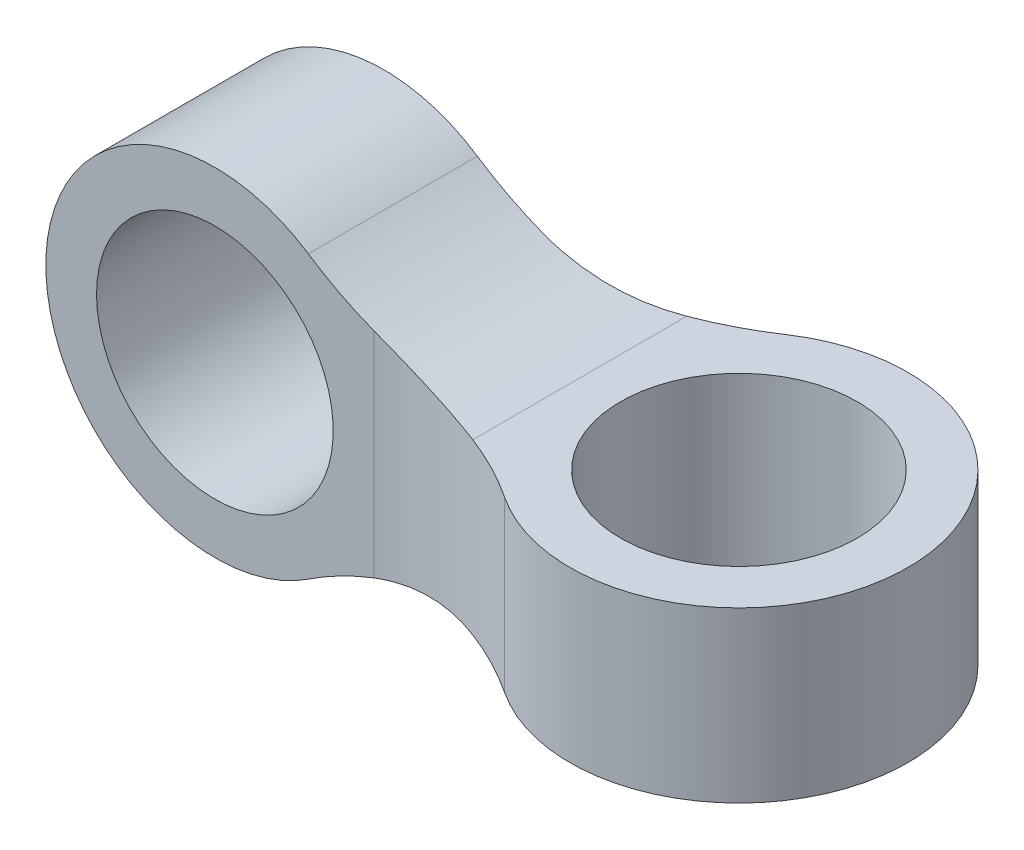
ISO-10303-21;
HEADER;
FILE_DESCRIPTION(('STEP AP214'),'2;1');
FILE_NAME('part.step','',(''),(''),'','','');
FILE_SCHEMA(('AUTOMOTIVE_DESIGN { 1 0 10303 214 1 1 1 1 }'));
ENDSEC;
DATA;
#1=APPLICATION_CONTEXT('core data for automotive mechanical design processes');
#2=APPLICATION_PROTOCOL_DEFINITION('international standard','automotive_design',2000,#1);
#3=PRODUCT_CONTEXT('',#1,'mechanical');
#4=PRODUCT('Part','Part','',(#3));
#5=PRODUCT_RELATED_PRODUCT_CATEGORY('part','',(#4));
#6=PRODUCT_DEFINITION_FORMATION('','',#4);
#7=PRODUCT_DEFINITION_CONTEXT('part definition',#1,'design');
#8=PRODUCT_DEFINITION('design','',#6,#7);
#9=PRODUCT_DEFINITION_SHAPE('','',#8);
#10=(LENGTH_UNIT() NAMED_UNIT(*) SI_UNIT(.MILLI.,.METRE.));
#11=(NAMED_UNIT(*) PLANE_ANGLE_UNIT() SI_UNIT($,.RADIAN.));
#12=(NAMED_UNIT(*) SI_UNIT($,.STERADIAN.) SOLID_ANGLE_UNIT());
#13=UNCERTAINTY_MEASURE_WITH_UNIT(LENGTH_MEASURE(1.E-05),#10,'distance_accuracy_value','');
#14=(GEOMETRIC_REPRESENTATION_CONTEXT(3) GLOBAL_UNCERTAINTY_ASSIGNED_CONTEXT((#13)) GLOBAL_UNIT_ASSIGNED_CONTEXT((#10,
#11,#12)) REPRESENTATION_CONTEXT('',''));
#15=CARTESIAN_POINT('',(0.,0.,0.));
#16=DIRECTION('',(0.,0.,1.));
#17=DIRECTION('',(1.,0.,0.));
#18=AXIS2_PLACEMENT_3D('',#15,#16,#17);
#19=CARTESIAN_POINT('',(-13.,0.,-25.));
#20=DIRECTION('',(0.,0.,1.));
#21=DIRECTION('',(1.,0.,0.));
#22=AXIS2_PLACEMENT_3D('',#19,#20,#21);
#23=CYLINDRICAL_SURFACE('',#22,10.);
#24=CARTESIAN_POINT('',(-13.,0.,5.));
#25=DIRECTION('',(0.,0.,-1.));
#26=DIRECTION('',(-1.,0.,0.));
#27=AXIS2_PLACEMENT_3D('',#24,#25,#26);
#28=CIRCLE('',#27,10.);
#29=CARTESIAN_POINT('',(-7.47229201607434,8.33333333333333,5.));
#30=VERTEX_POINT('',#29);
#31=CARTESIAN_POINT('',(-7.47229201607434,-8.33333333333333,5.));
#32=VERTEX_POINT('',#31);
#33=EDGE_CURVE('E345',#30,#32,#28,.F.);
#34=ORIENTED_EDGE('',*,*,#33,.F.);
#35=DIRECTION('',(0.,0.,1.));
#36=VECTOR('',#35,1.);
#37=CARTESIAN_POINT('',(-7.47229201607434,8.33333333333333,-25.));
#38=LINE('',#37,#36);
#39=CARTESIAN_POINT('',(-7.47229201607434,8.33333333333333,-5.));
#40=VERTEX_POINT('',#39);
#41=EDGE_CURVE('E310',#40,#30,#38,.T.);
#42=ORIENTED_EDGE('',*,*,#41,.F.);
#43=CARTESIAN_POINT('',(-13.,0.,-5.));
#44=DIRECTION('',(0.,0.,-1.));
#45=DIRECTION('',(-1.,0.,0.));
#46=AXIS2_PLACEMENT_3D('',#43,#44,#45);
#47=CIRCLE('',#46,10.);
#48=CARTESIAN_POINT('',(-7.47229201607434,-8.33333333333333,-5.));
#49=VERTEX_POINT('',#48);
#50=EDGE_CURVE('E233',#40,#49,#47,.F.);
#51=ORIENTED_EDGE('',*,*,#50,.T.);
#52=DIRECTION('',(0.,0.,1.));
#53=VECTOR('',#52,1.);
#54=CARTESIAN_POINT('',(-7.47229201607434,-8.33333333333333,-25.));
#55=LINE('',#54,#53);
#56=EDGE_CURVE('E301',#49,#32,#55,.T.);
#57=ORIENTED_EDGE('',*,*,#56,.T.);
#58=EDGE_LOOP('',(#34,#42,#51,#57));
#59=FACE_BOUND('',#58,.T.);
#60=ADVANCED_FACE('F165',(#59),#23,.T.);
#61=CARTESIAN_POINT('',(0.,5.,-25.));
#62=DIRECTION('',(0.,-1.,0.));
#63=DIRECTION('',(1.,0.,0.));
#64=AXIS2_PLACEMENT_3D('',#61,#62,#63);
#65=PLANE('',#64);
#66=CARTESIAN_POINT('',(13.,5.,0.));
#67=DIRECTION('',(0.,-1.,0.));
#68=DIRECTION('',(1.,0.,0.));
#69=AXIS2_PLACEMENT_3D('',#66,#67,#68);
#70=CIRCLE('',#69,7.);
#71=CARTESIAN_POINT('',(20.,5.,0.));
#72=VERTEX_POINT('',#71);
#73=EDGE_CURVE('E324',#72,#72,#70,.T.);
#74=ORIENTED_EDGE('',*,*,#73,.T.);
#75=EDGE_LOOP('',(#74));
#76=FACE_BOUND('',#75,.T.);
#77=CARTESIAN_POINT('',(-3.583123951777,5.,25.));
#78=DIRECTION('',(0.,-1.,0.));
#79=DIRECTION('',(1.,0.,0.));
#80=AXIS2_PLACEMENT_3D('',#77,#78,#79);
#81=CIRCLE('',#80,20.);
#82=CARTESIAN_POINT('',(7.47229201607434,5.,8.33333333333334));
#83=VERTEX_POINT('',#82);
#84=CARTESIAN_POINT('',(3.58312395177704,4.99999999999995,6.32796500151069));
#85=VERTEX_POINT('',#84);
#86=EDGE_CURVE('E177',#83,#85,#81,.F.);
#87=ORIENTED_EDGE('',*,*,#86,.F.);
#88=CARTESIAN_POINT('',(13.,5.,0.));
#89=DIRECTION('',(0.,-1.,0.));
#90=DIRECTION('',(1.,0.,0.));
#91=AXIS2_PLACEMENT_3D('',#88,#89,#90);
#92=CIRCLE('',#91,10.);
#93=CARTESIAN_POINT('',(7.47229201607433,5.,-8.33333333333333));
#94=VERTEX_POINT('',#93);
#95=EDGE_CURVE('E256',#94,#83,#92,.T.);
#96=ORIENTED_EDGE('',*,*,#95,.F.);
#97=CARTESIAN_POINT('',(-3.583123951777,5.,-25.));
#98=DIRECTION('',(0.,-1.,0.));
#99=DIRECTION('',(1.,0.,0.));
#100=AXIS2_PLACEMENT_3D('',#97,#98,#99);
#101=CIRCLE('',#100,20.);
#102=CARTESIAN_POINT('',(3.58312395177704,4.99999999999995,-6.32796500151069));
#103=VERTEX_POINT('',#102);
#104=EDGE_CURVE('E254',#94,#103,#101,.T.);
#105=ORIENTED_EDGE('',*,*,#104,.T.);
#106=DIRECTION('',(0.,0.,1.));
#107=VECTOR('',#106,1.);
#108=CARTESIAN_POINT('',(3.58312395177699,5.,-25.));
#109=LINE('',#108,#107);
#110=EDGE_CURVE('E255',#103,#85,#109,.T.);
#111=ORIENTED_EDGE('',*,*,#110,.T.);
#112=EDGE_LOOP('',(#87,#96,#105,#111));
#113=FACE_BOUND('',#112,.T.);
#114=ADVANCED_FACE('F349',(#76,#113),#65,.F.);
#115=CARTESIAN_POINT('',(3.58312395177699,25.,-25.));
#116=DIRECTION('',(0.,0.,1.));
#117=DIRECTION('',(1.,0.,0.));
#118=AXIS2_PLACEMENT_3D('',#115,#116,#117);
#119=CYLINDRICAL_SURFACE('',#118,20.);
#120=CARTESIAN_POINT('',(7.47229201607434,5.38178469463521,8.33333333333333));
#121=CARTESIAN_POINT('',(7.29699032317259,5.34703236946405,8.21705135141738));
#122=CARTESIAN_POINT('',(7.11958800828395,5.31430622195632,8.10335941718668));
#123=CARTESIAN_POINT('',(6.76071891900881,5.2532019543182,7.88131271793948));
#124=CARTESIAN_POINT('',(6.57925177284516,5.22482423377966,7.7729584440389));
#125=CARTESIAN_POINT('',(6.02882561809351,5.14664056772693,7.45606457285716));
#126=CARTESIAN_POINT('',(5.6540157645712,5.1038191206325,7.25580939391501));
#127=CARTESIAN_POINT('',(4.88995933117876,5.03904902020734,6.8784966546735));
#128=CARTESIAN_POINT('',(4.50067842728979,5.01715378266823,6.70149944909328));
#129=CARTESIAN_POINT('',(3.71110175343317,4.99651277313733,6.37267960841244));
#130=CARTESIAN_POINT('',(3.31080898852315,4.99776074689242,6.22085018312637));
#131=CARTESIAN_POINT('',(2.50015157937633,5.02520585072317,5.94276436337308));
#132=CARTESIAN_POINT('',(2.08974859443147,5.05151960391396,5.81663085531488));
#133=CARTESIAN_POINT('',(1.26396259082839,5.13058788823112,5.59152465950283));
#134=CARTESIAN_POINT('',(0.848578641653094,5.18334743736802,5.49255713193));
#135=CARTESIAN_POINT('',(0.0177355960030123,5.31588247949777,5.3222677787619));
#136=CARTESIAN_POINT('',(-0.397719870811708,5.39558008538139,5.25086750767909));
#137=CARTESIAN_POINT('',(-1.22607394668929,5.58218052923217,5.13497842084868));
#138=CARTESIAN_POINT('',(-1.63897376743929,5.68906927003721,5.09047570038574));
#139=CARTESIAN_POINT('',(-2.30757201952622,5.88528115160457,5.03902874204332));
#140=CARTESIAN_POINT('',(-2.56509330773308,5.96654705369896,5.02428612595834));
#141=CARTESIAN_POINT('',(-3.07676594844552,6.13949048658364,5.00477143854931));
#142=CARTESIAN_POINT('',(-3.33091988173299,6.23115945884189,4.99999123302929));
#143=CARTESIAN_POINT('',(-3.583123951777,6.32796500151074,5.));
#144=B_SPLINE_CURVE_WITH_KNOTS('',3,(#120,#121,#122,#123,#124,#125,#126,#127,#128,#129,#130,
#131,#132,#133,#134,#135,#136,#137,#138,#139,#140,#141,#142,#143),.UNSPECIFIED.,.F.,.F.,(4,2,2,
2,2,2,2,2,2,2,2,4),(0.,0.639568646578073,1.27919603010921,2.55908404816412,3.84223042353997,
5.12503004473554,6.41382742723958,7.70286944781018,8.98821584478183,10.2728972110752,
11.083848336485,11.8941370696184),.UNSPECIFIED.);
#145=CARTESIAN_POINT('',(-3.583123951777,6.32796500151074,5.));
#146=VERTEX_POINT('',#145);
#147=EDGE_CURVE('E296',#85,#146,#144,.T.);
#148=ORIENTED_EDGE('',*,*,#147,.F.);
#149=ORIENTED_EDGE('',*,*,#110,.F.);
#150=CARTESIAN_POINT('',(7.47229201607433,5.3817846946352,-8.33333333333334));
#151=CARTESIAN_POINT('',(7.29699032317258,5.34703236946404,-8.21705135141739));
#152=CARTESIAN_POINT('',(7.11958800828394,5.31430622195631,-8.10335941718669));
#153=CARTESIAN_POINT('',(6.7607189190088,5.2532019543182,-7.88131271793948));
#154=CARTESIAN_POINT('',(6.57925177284515,5.22482423377965,-7.7729584440389));
#155=CARTESIAN_POINT('',(6.0288256180935,5.14664056772693,-7.45606457285716));
#156=CARTESIAN_POINT('',(5.6540157645712,5.1038191206325,-7.25580939391501));
#157=CARTESIAN_POINT('',(4.88995933117876,5.03904902020734,-6.8784966546735));
#158=CARTESIAN_POINT('',(4.50067842728979,5.01715378266822,-6.70149944909328));
#159=CARTESIAN_POINT('',(3.71110175343317,4.99651277313733,-6.37267960841245));
#160=CARTESIAN_POINT('',(3.31080898852315,4.99776074689242,-6.22085018312637));
#161=CARTESIAN_POINT('',(2.50015157937632,5.02520585072317,-5.94276436337308));
#162=CARTESIAN_POINT('',(2.08974859443147,5.05151960391397,-5.81663085531489));
#163=CARTESIAN_POINT('',(1.26396259082839,5.13058788823112,-5.59152465950283));
#164=CARTESIAN_POINT('',(0.848578641653089,5.18334743736802,-5.49255713193001));
#165=CARTESIAN_POINT('',(0.0177355960030073,5.31588247949777,-5.3222677787619));
#166=CARTESIAN_POINT('',(-0.397719870811712,5.39558008538139,-5.25086750767909));
#167=CARTESIAN_POINT('',(-1.22607394668929,5.58218052923217,-5.13497842084869));
#168=CARTESIAN_POINT('',(-1.63897376743929,5.68906927003722,-5.09047570038574));
#169=CARTESIAN_POINT('',(-2.30757201952623,5.88528115160457,-5.03902874204333));
#170=CARTESIAN_POINT('',(-2.56509330773309,5.96654705369896,-5.02428612595834));
#171=CARTESIAN_POINT('',(-3.07676594844552,6.13949048658364,-5.00477143854931));
#172=CARTESIAN_POINT('',(-3.330919881733,6.23115945884189,-4.9999912330293));
#173=CARTESIAN_POINT('',(-3.583123951777,6.32796500151074,-5.));
#174=B_SPLINE_CURVE_WITH_KNOTS('',3,(#150,#151,#152,#153,#154,#155,#156,#157,#158,#159,#160,
#161,#162,#163,#164,#165,#166,#167,#168,#169,#170,#171,#172,#173),.UNSPECIFIED.,.F.,.F.,(4,2,2,
2,2,2,2,2,2,2,2,4),(0.,0.639568646578075,1.27919603010921,2.55908404816412,3.84223042353997,
5.12503004473554,6.41382742723958,7.70286944781018,8.98821584478183,10.2728972110752,
11.083848336485,11.8941370696184),.UNSPECIFIED.);
#175=CARTESIAN_POINT('',(-3.583123951777,6.32796500151074,-5.));
#176=VERTEX_POINT('',#175);
#177=EDGE_CURVE('E244',#103,#176,#174,.T.);
#178=ORIENTED_EDGE('',*,*,#177,.T.);
#179=CARTESIAN_POINT('',(3.58312395177699,25.,-5.));
#180=DIRECTION('',(0.,0.,-1.));
#181=DIRECTION('',(-1.,0.,0.));
#182=AXIS2_PLACEMENT_3D('',#179,#180,#181);
#183=CIRCLE('',#182,20.);
#184=EDGE_CURVE('E230',#40,#176,#183,.F.);
#185=ORIENTED_EDGE('',*,*,#184,.F.);
#186=ORIENTED_EDGE('',*,*,#41,.T.);
#187=CARTESIAN_POINT('',(3.58312395177699,25.,5.));
#188=DIRECTION('',(0.,0.,-1.));
#189=DIRECTION('',(-1.,0.,0.));
#190=AXIS2_PLACEMENT_3D('',#187,#188,#189);
#191=CIRCLE('',#190,20.);
#192=EDGE_CURVE('E326',#30,#146,#191,.F.);
#193=ORIENTED_EDGE('',*,*,#192,.T.);
#194=EDGE_LOOP('',(#148,#149,#178,#185,#186,#193));
#195=FACE_BOUND('',#194,.T.);
#196=ADVANCED_FACE('F252',(#195),#119,.F.);
#197=CARTESIAN_POINT('',(3.583123951777,-25.,-25.));
#198=DIRECTION('',(0.,0.,1.));
#199=DIRECTION('',(1.,0.,0.));
#200=AXIS2_PLACEMENT_3D('',#197,#198,#199);
#201=CYLINDRICAL_SURFACE('',#200,20.);
#202=DIRECTION('',(0.,0.,1.));
#203=VECTOR('',#202,1.);
#204=CARTESIAN_POINT('',(3.583123951777,-5.,-25.));
#205=LINE('',#204,#203);
#206=CARTESIAN_POINT('',(3.583123951777,-5.,-6.32796500151074));
#207=VERTEX_POINT('',#206);
#208=CARTESIAN_POINT('',(3.583123951777,-5.,6.32796500151073));
#209=VERTEX_POINT('',#208);
#210=EDGE_CURVE('E308',#207,#209,#205,.T.);
#211=ORIENTED_EDGE('',*,*,#210,.T.);
#212=CARTESIAN_POINT('',(7.47229201607434,-5.3817846946352,8.33333333333333));
#213=CARTESIAN_POINT('',(7.29699032317258,-5.34703236946403,8.21705135141738));
#214=CARTESIAN_POINT('',(7.11958800828395,-5.31430622195631,8.10335941718668));
#215=CARTESIAN_POINT('',(6.7607189190088,-5.25320195431819,7.88131271793948));
#216=CARTESIAN_POINT('',(6.57925177284515,-5.22482423377964,7.7729584440389));
#217=CARTESIAN_POINT('',(6.02882561809351,-5.14664056772692,7.45606457285716));
#218=CARTESIAN_POINT('',(5.6540157645712,-5.10381912063249,7.25580939391501));
#219=CARTESIAN_POINT('',(4.88995933117876,-5.03904902020733,6.87849665467349));
#220=CARTESIAN_POINT('',(4.50067842728979,-5.01715378266822,6.70149944909328));
#221=CARTESIAN_POINT('',(3.71110175343317,-4.99651277313733,6.37267960841245));
#222=CARTESIAN_POINT('',(3.31080898852315,-4.99776074689242,6.22085018312637));
#223=CARTESIAN_POINT('',(2.50015157937633,-5.02520585072316,5.94276436337308));
#224=CARTESIAN_POINT('',(2.08974859443147,-5.05151960391396,5.81663085531488));
#225=CARTESIAN_POINT('',(1.26396259082839,-5.13058788823111,5.59152465950283));
#226=CARTESIAN_POINT('',(0.848578641653091,-5.18334743736801,5.49255713193));
#227=CARTESIAN_POINT('',(0.0177355960030095,-5.31588247949776,5.3222677787619));
#228=CARTESIAN_POINT('',(-0.39771987081171,-5.39558008538138,5.25086750767909));
#229=CARTESIAN_POINT('',(-1.22607394668929,-5.58218052923217,5.13497842084868));
#230=CARTESIAN_POINT('',(-1.63897376743929,-5.68906927003721,5.09047570038574));
#231=CARTESIAN_POINT('',(-2.30757201952623,-5.88528115160457,5.03902874204332));
#232=CARTESIAN_POINT('',(-2.56509330773309,-5.96654705369895,5.02428612595834));
#233=CARTESIAN_POINT('',(-3.07676594844552,-6.13949048658363,5.00477143854931));
#234=CARTESIAN_POINT('',(-3.33091988173299,-6.23115945884189,4.99999123302929));
#235=CARTESIAN_POINT('',(-3.583123951777,-6.32796500151074,5.));
#236=B_SPLINE_CURVE_WITH_KNOTS('',3,(#212,#213,#214,#215,#216,#217,#218,#219,#220,#221,#222,
#223,#224,#225,#226,#227,#228,#229,#230,#231,#232,#233,#234,#235),.UNSPECIFIED.,.F.,.F.,(4,2,2,
2,2,2,2,2,2,2,2,4),(0.,0.639568646578074,1.27919603010921,2.55908404816412,3.84223042353997,
5.12503004473554,6.41382742723958,7.70286944781018,8.98821584478183,10.2728972110752,
11.083848336485,11.8941370696184),.UNSPECIFIED.);
#237=CARTESIAN_POINT('',(-3.583123951777,-6.32796500151073,5.));
#238=VERTEX_POINT('',#237);
#239=EDGE_CURVE('E181',#209,#238,#236,.T.);
#240=ORIENTED_EDGE('',*,*,#239,.T.);
#241=CARTESIAN_POINT('',(3.583123951777,-25.,5.));
#242=DIRECTION('',(0.,0.,-1.));
#243=DIRECTION('',(-1.,0.,0.));
#244=AXIS2_PLACEMENT_3D('',#241,#242,#243);
#245=CIRCLE('',#244,20.);
#246=EDGE_CURVE('E321',#32,#238,#245,.T.);
#247=ORIENTED_EDGE('',*,*,#246,.F.);
#248=ORIENTED_EDGE('',*,*,#56,.F.);
#249=CARTESIAN_POINT('',(3.583123951777,-25.,-5.));
#250=DIRECTION('',(0.,0.,-1.));
#251=DIRECTION('',(-1.,0.,0.));
#252=AXIS2_PLACEMENT_3D('',#249,#250,#251);
#253=CIRCLE('',#252,20.);
#254=CARTESIAN_POINT('',(-3.583123951777,-6.32796500151074,-5.));
#255=VERTEX_POINT('',#254);
#256=EDGE_CURVE('E318',#49,#255,#253,.T.);
#257=ORIENTED_EDGE('',*,*,#256,.T.);
#258=CARTESIAN_POINT('',(7.47229201607433,-5.3817846946352,-8.33333333333334));
#259=CARTESIAN_POINT('',(7.29699032317258,-5.34703236946403,-8.21705135141739));
#260=CARTESIAN_POINT('',(7.11958800828394,-5.3143062219563,-8.10335941718669));
#261=CARTESIAN_POINT('',(6.7607189190088,-5.25320195431819,-7.88131271793948));
#262=CARTESIAN_POINT('',(6.57925177284515,-5.22482423377964,-7.7729584440389));
#263=CARTESIAN_POINT('',(6.0288256180935,-5.14664056772692,-7.45606457285716));
#264=CARTESIAN_POINT('',(5.6540157645712,-5.10381912063249,-7.25580939391501));
#265=CARTESIAN_POINT('',(4.88995933117876,-5.03904902020733,-6.8784966546735));
#266=CARTESIAN_POINT('',(4.50067842728978,-5.01715378266822,-6.70149944909328));
#267=CARTESIAN_POINT('',(3.71110175343316,-4.99651277313732,-6.37267960841245));
#268=CARTESIAN_POINT('',(3.31080898852314,-4.99776074689241,-6.22085018312637));
#269=CARTESIAN_POINT('',(2.50015157937632,-5.02520585072316,-5.94276436337308));
#270=CARTESIAN_POINT('',(2.08974859443146,-5.05151960391396,-5.81663085531489));
#271=CARTESIAN_POINT('',(1.26396259082838,-5.13058788823111,-5.59152465950283));
#272=CARTESIAN_POINT('',(0.848578641653084,-5.18334743736801,-5.49255713193001));
#273=CARTESIAN_POINT('',(0.0177355960030023,-5.31588247949776,-5.3222677787619));
#274=CARTESIAN_POINT('',(-0.397719870811718,-5.39558008538138,-5.25086750767909));
#275=CARTESIAN_POINT('',(-1.2260739466893,-5.58218052923217,-5.13497842084869));
#276=CARTESIAN_POINT('',(-1.6389737674393,-5.68906927003721,-5.09047570038574));
#277=CARTESIAN_POINT('',(-2.30757201952623,-5.88528115160457,-5.03902874204333));
#278=CARTESIAN_POINT('',(-2.56509330773309,-5.96654705369895,-5.02428612595834));
#279=CARTESIAN_POINT('',(-3.07676594844552,-6.13949048658363,-5.00477143854931));
#280=CARTESIAN_POINT('',(-3.330919881733,-6.23115945884188,-4.9999912330293));
#281=CARTESIAN_POINT('',(-3.583123951777,-6.32796500151074,-5.));
#282=B_SPLINE_CURVE_WITH_KNOTS('',3,(#258,#259,#260,#261,#262,#263,#264,#265,#266,#267,#268,
#269,#270,#271,#272,#273,#274,#275,#276,#277,#278,#279,#280,#281),.UNSPECIFIED.,.F.,.F.,(4,2,2,
2,2,2,2,2,2,2,2,4),(0.,0.639568646578075,1.27919603010921,2.55908404816412,3.84223042353997,
5.12503004473554,6.41382742723958,7.70286944781018,8.98821584478183,10.2728972110752,
11.083848336485,11.8941370696184),.UNSPECIFIED.);
#283=EDGE_CURVE('E250',#207,#255,#282,.T.);
#284=ORIENTED_EDGE('',*,*,#283,.F.);
#285=EDGE_LOOP('',(#211,#240,#247,#248,#257,#284));
#286=FACE_BOUND('',#285,.T.);
#287=ADVANCED_FACE('F335',(#286),#201,.F.);
#288=CARTESIAN_POINT('',(0.,-5.,-25.));
#289=DIRECTION('',(0.,-1.,0.));
#290=DIRECTION('',(1.,0.,0.));
#291=AXIS2_PLACEMENT_3D('',#288,#289,#290);
#292=PLANE('',#291);
#293=CARTESIAN_POINT('',(13.,-5.,0.));
#294=DIRECTION('',(0.,-1.,0.));
#295=DIRECTION('',(1.,0.,0.));
#296=AXIS2_PLACEMENT_3D('',#293,#294,#295);
#297=CIRCLE('',#296,7.);
#298=CARTESIAN_POINT('',(20.,-5.,0.));
#299=VERTEX_POINT('',#298);
#300=EDGE_CURVE('E325',#299,#299,#297,.T.);
#301=ORIENTED_EDGE('',*,*,#300,.F.);
#302=EDGE_LOOP('',(#301));
#303=FACE_BOUND('',#302,.T.);
#304=CARTESIAN_POINT('',(13.,-5.,0.));
#305=DIRECTION('',(0.,-1.,0.));
#306=DIRECTION('',(1.,0.,0.));
#307=AXIS2_PLACEMENT_3D('',#304,#305,#306);
#308=CIRCLE('',#307,10.);
#309=CARTESIAN_POINT('',(7.47229201607433,-5.,-8.33333333333333));
#310=VERTEX_POINT('',#309);
#311=CARTESIAN_POINT('',(7.47229201607434,-5.,8.33333333333334));
#312=VERTEX_POINT('',#311);
#313=EDGE_CURVE('E311',#310,#312,#308,.T.);
#314=ORIENTED_EDGE('',*,*,#313,.T.);
#315=CARTESIAN_POINT('',(-3.583123951777,-5.,25.));
#316=DIRECTION('',(0.,-1.,0.));
#317=DIRECTION('',(1.,0.,0.));
#318=AXIS2_PLACEMENT_3D('',#315,#316,#317);
#319=CIRCLE('',#318,20.);
#320=EDGE_CURVE('E12',#312,#209,#319,.F.);
#321=ORIENTED_EDGE('',*,*,#320,.T.);
#322=ORIENTED_EDGE('',*,*,#210,.F.);
#323=CARTESIAN_POINT('',(-3.583123951777,-5.,-25.));
#324=DIRECTION('',(0.,-1.,0.));
#325=DIRECTION('',(1.,0.,0.));
#326=AXIS2_PLACEMENT_3D('',#323,#324,#325);
#327=CIRCLE('',#326,20.);
#328=EDGE_CURVE('E166',#310,#207,#327,.T.);
#329=ORIENTED_EDGE('',*,*,#328,.F.);
#330=EDGE_LOOP('',(#314,#321,#322,#329));
#331=FACE_BOUND('',#330,.T.);
#332=ADVANCED_FACE('F289',(#303,#331),#292,.T.);
#333=CARTESIAN_POINT('',(-3.583123951777,30.,25.));
#334=DIRECTION('',(0.,-1.,0.));
#335=DIRECTION('',(1.,0.,0.));
#336=AXIS2_PLACEMENT_3D('',#333,#334,#335);
#337=CYLINDRICAL_SURFACE('',#336,20.);
#338=ORIENTED_EDGE('',*,*,#86,.T.);
#339=ORIENTED_EDGE('',*,*,#147,.T.);
#340=DIRECTION('',(0.,-1.,0.));
#341=VECTOR('',#340,1.);
#342=CARTESIAN_POINT('',(-3.583123951777,30.,5.));
#343=LINE('',#342,#341);
#344=EDGE_CURVE('E248',#146,#238,#343,.T.);
#345=ORIENTED_EDGE('',*,*,#344,.T.);
#346=ORIENTED_EDGE('',*,*,#239,.F.);
#347=ORIENTED_EDGE('',*,*,#320,.F.);
#348=DIRECTION('',(0.,-1.,0.));
#349=VECTOR('',#348,1.);
#350=CARTESIAN_POINT('',(7.47229201607434,30.,8.33333333333334));
#351=LINE('',#350,#349);
#352=EDGE_CURVE('E333',#83,#312,#351,.T.);
#353=ORIENTED_EDGE('',*,*,#352,.F.);
#354=EDGE_LOOP('',(#338,#339,#345,#346,#347,#353));
#355=FACE_BOUND('',#354,.T.);
#356=ADVANCED_FACE('F276',(#355),#337,.F.);
#357=CARTESIAN_POINT('',(-3.583123951777,30.,-25.));
#358=DIRECTION('',(0.,-1.,0.));
#359=DIRECTION('',(1.,0.,0.));
#360=AXIS2_PLACEMENT_3D('',#357,#358,#359);
#361=CYLINDRICAL_SURFACE('',#360,20.);
#362=DIRECTION('',(0.,-1.,0.));
#363=VECTOR('',#362,1.);
#364=CARTESIAN_POINT('',(7.47229201607433,30.,-8.33333333333333));
#365=LINE('',#364,#363);
#366=EDGE_CURVE('E249',#94,#310,#365,.T.);
#367=ORIENTED_EDGE('',*,*,#366,.T.);
#368=ORIENTED_EDGE('',*,*,#328,.T.);
#369=ORIENTED_EDGE('',*,*,#283,.T.);
#370=DIRECTION('',(0.,-1.,0.));
#371=VECTOR('',#370,1.);
#372=CARTESIAN_POINT('',(-3.583123951777,30.,-5.));
#373=LINE('',#372,#371);
#374=EDGE_CURVE('E232',#176,#255,#373,.T.);
#375=ORIENTED_EDGE('',*,*,#374,.F.);
#376=ORIENTED_EDGE('',*,*,#177,.F.);
#377=ORIENTED_EDGE('',*,*,#104,.F.);
#378=EDGE_LOOP('',(#367,#368,#369,#375,#376,#377));
#379=FACE_BOUND('',#378,.T.);
#380=ADVANCED_FACE('F245',(#379),#361,.F.);
#381=CARTESIAN_POINT('',(13.,30.,0.));
#382=DIRECTION('',(0.,-1.,0.));
#383=DIRECTION('',(1.,0.,0.));
#384=AXIS2_PLACEMENT_3D('',#381,#382,#383);
#385=CYLINDRICAL_SURFACE('',#384,10.);
#386=ORIENTED_EDGE('',*,*,#366,.F.);
#387=ORIENTED_EDGE('',*,*,#95,.T.);
#388=ORIENTED_EDGE('',*,*,#352,.T.);
#389=ORIENTED_EDGE('',*,*,#313,.F.);
#390=EDGE_LOOP('',(#386,#387,#388,#389));
#391=FACE_BOUND('',#390,.T.);
#392=ADVANCED_FACE('F279',(#391),#385,.T.);
#393=CARTESIAN_POINT('',(0.,30.,5.));
#394=DIRECTION('',(0.,0.,-1.));
#395=DIRECTION('',(-1.,0.,0.));
#396=AXIS2_PLACEMENT_3D('',#393,#394,#395);
#397=PLANE('',#396);
#398=CARTESIAN_POINT('',(-13.,0.,5.));
#399=DIRECTION('',(0.,0.,-1.));
#400=DIRECTION('',(-1.,0.,0.));
#401=AXIS2_PLACEMENT_3D('',#398,#399,#400);
#402=CIRCLE('',#401,7.);
#403=CARTESIAN_POINT('',(-20.,0.,5.));
#404=VERTEX_POINT('',#403);
#405=EDGE_CURVE('E236',#404,#404,#402,.F.);
#406=ORIENTED_EDGE('',*,*,#405,.F.);
#407=EDGE_LOOP('',(#406));
#408=FACE_BOUND('',#407,.T.);
#409=ORIENTED_EDGE('',*,*,#192,.F.);
#410=ORIENTED_EDGE('',*,*,#33,.T.);
#411=ORIENTED_EDGE('',*,*,#246,.T.);
#412=ORIENTED_EDGE('',*,*,#344,.F.);
#413=EDGE_LOOP('',(#409,#410,#411,#412));
#414=FACE_BOUND('',#413,.T.);
#415=ADVANCED_FACE('F284',(#408,#414),#397,.F.);
#416=CARTESIAN_POINT('',(0.,30.,-5.));
#417=DIRECTION('',(0.,0.,-1.));
#418=DIRECTION('',(-1.,0.,0.));
#419=AXIS2_PLACEMENT_3D('',#416,#417,#418);
#420=PLANE('',#419);
#421=CARTESIAN_POINT('',(-13.,0.,-5.));
#422=DIRECTION('',(0.,0.,-1.));
#423=DIRECTION('',(-1.,0.,0.));
#424=AXIS2_PLACEMENT_3D('',#421,#422,#423);
#425=CIRCLE('',#424,7.);
#426=CARTESIAN_POINT('',(-20.,0.,-5.));
#427=VERTEX_POINT('',#426);
#428=EDGE_CURVE('E312',#427,#427,#425,.F.);
#429=ORIENTED_EDGE('',*,*,#428,.T.);
#430=EDGE_LOOP('',(#429));
#431=FACE_BOUND('',#430,.T.);
#432=ORIENTED_EDGE('',*,*,#184,.T.);
#433=ORIENTED_EDGE('',*,*,#374,.T.);
#434=ORIENTED_EDGE('',*,*,#256,.F.);
#435=ORIENTED_EDGE('',*,*,#50,.F.);
#436=EDGE_LOOP('',(#432,#433,#434,#435));
#437=FACE_BOUND('',#436,.T.);
#438=ADVANCED_FACE('F229',(#431,#437),#420,.T.);
#439=CARTESIAN_POINT('',(13.,30.,0.));
#440=DIRECTION('',(0.,-1.,0.));
#441=DIRECTION('',(1.,0.,0.));
#442=AXIS2_PLACEMENT_3D('',#439,#440,#441);
#443=CYLINDRICAL_SURFACE('',#442,7.);
#444=ORIENTED_EDGE('',*,*,#300,.T.);
#445=EDGE_LOOP('',(#444));
#446=FACE_BOUND('',#445,.T.);
#447=ORIENTED_EDGE('',*,*,#73,.F.);
#448=EDGE_LOOP('',(#447));
#449=FACE_BOUND('',#448,.T.);
#450=ADVANCED_FACE('F286',(#446,#449),#443,.F.);
#451=CARTESIAN_POINT('',(-13.,0.,-25.));
#452=DIRECTION('',(0.,0.,1.));
#453=DIRECTION('',(1.,0.,0.));
#454=AXIS2_PLACEMENT_3D('',#451,#452,#453);
#455=CYLINDRICAL_SURFACE('',#454,7.);
#456=ORIENTED_EDGE('',*,*,#405,.T.);
#457=EDGE_LOOP('',(#456));
#458=FACE_BOUND('',#457,.T.);
#459=ORIENTED_EDGE('',*,*,#428,.F.);
#460=EDGE_LOOP('',(#459));
#461=FACE_BOUND('',#460,.T.);
#462=ADVANCED_FACE('F351',(#458,#461),#455,.F.);
#463=CLOSED_SHELL('',(#60,#114,#196,#287,#332,#356,#380,#392,#415,#438,#450,#462));
#464=MANIFOLD_SOLID_BREP('B2',#463);
#465=ADVANCED_BREP_SHAPE_REPRESENTATION('',(#18,#464),#14);
#466=SHAPE_DEFINITION_REPRESENTATION(#9,#465);
ENDSEC;
END-ISO-10303-21;
